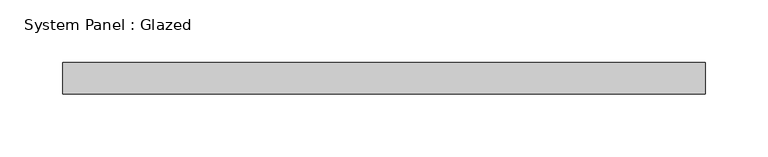
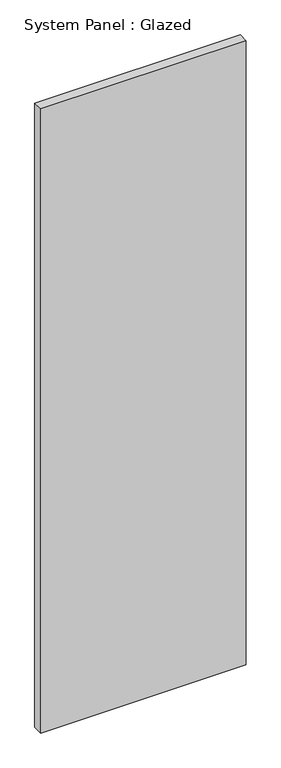
"""IFC4 building model written with IfcOpenShell, lengths in millimetres: plate geometry, System Panel : Glazed."""

from ifc_helpers import new_model, si_unit, origin, origin_with_axes, place, context, project, spatial, polyline, outline, extrude, source, transform, mapped, element, save


def system_panel_glazed_b01bb026(model_context):
    return source(origin(), model_context, "Body", "SweptSolid", [
        extrude(outline(polyline([(257.175, 19.05), (-257.175, 19.05), (-257.175, 44.45), (257.175, 44.45), (257.175, 19.05)])), origin_with_axes(), (0.0, 0.0, 1.0), 1650.3307027),
    ])


if __name__ == "__main__":
    model = new_model("IFC4")
    model_context = context("Model", 3, world=origin())
    ifc_project = project(units=[si_unit("LENGTHUNIT", "METRE", prefix="MILLI")], contexts=[model_context])
    site = spatial("IfcSite", under=ifc_project)
    building = spatial("IfcBuilding", under=site)
    placement = place(None, origin())
    system_panel_glazed_shape = system_panel_glazed_b01bb026(model_context)
    element("IfcPlate", 1, ObjectType="System Panel : Glazed", at=placement, inside=building, context=model_context, shape_type="MappedRepresentation", body=[
        mapped(system_panel_glazed_shape, transform((0.0, 0.0, 0.0), x_axis=(1.0, 0.0, 0.0), y_axis=(0.0, 1.0, 0.0), z_axis=(0.0, 0.0, 1.0))),
    ])
    save(model, "model.ifc")

# Revit data of these elements
# Type "System Panel : Glazed"
#   Construction Type Id = "GSP4R"
#   Analytic Construction = "1/8 in Pilkington single glazing"
#   Visual Light Transmittance = 0.9
#   Solar Heat Gain Coefficient = 0.86
#   Heat Transfer Coefficient (U) = 1.18115 BTU/(h·ft²·°F)
#   Define Thermal Properties by = 1
# Element 1 (IfcPlate, "System Panel : Glazed")
#   Materials on its faces: "Glass"
# Materials
#   "Glass": class "Glass", colour RGB 0 128 192, transparency 0.75, Description = "Soda Lime Glass", Cost = 0
